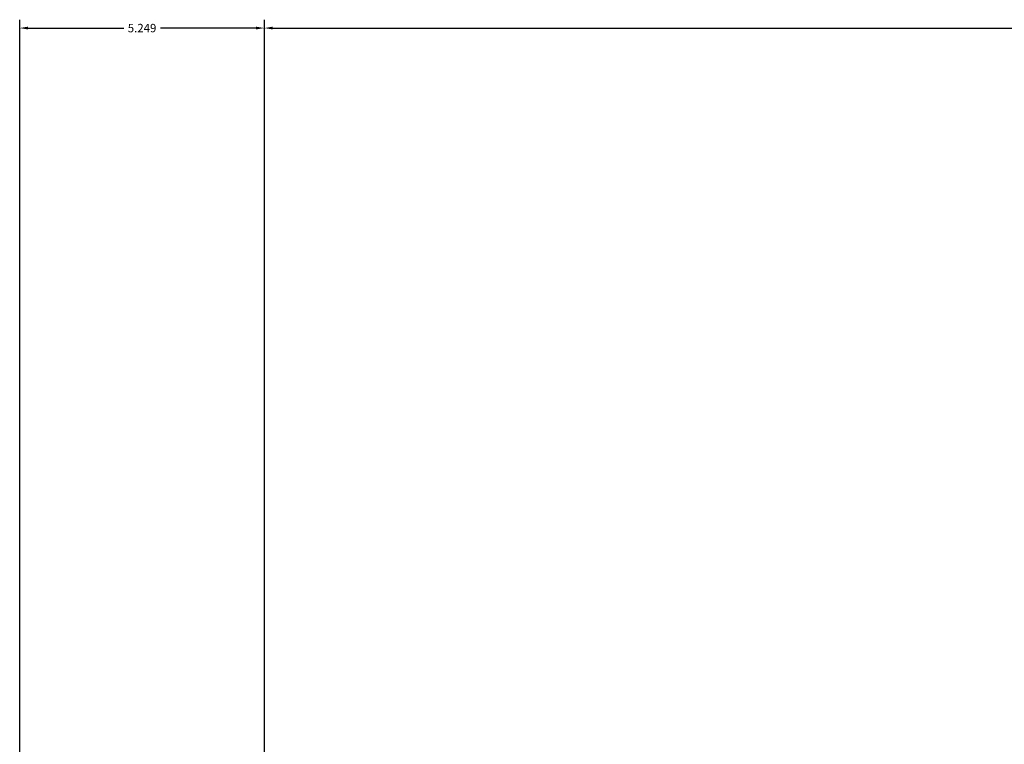
# Model space of a CAD drawing. Units: feet. Extents: x 2695 to 2912, y 795 to 1139.
# Tile 50 of 83: x 2711 to 2732, y 1123 to 1139. Entities that reach past the tile are written whole.
import ezdxf

# ---------------------------------------------------------------- set-up
doc = ezdxf.new("R2010")
doc.units = ezdxf.units.FT
doc.layers.add('A-ANNO-DIMS', color=2, linetype='Continuous', lineweight=18)
doc.styles.get("Standard").update_dxf_attribs({"font": 'arial.ttf'})
doc.dimstyles.get("Standard").update_dxf_attribs({"dimtxt": 0.18, "dimasz": 0.18, "dimexe": 0.18, "dimexo": 0.0625, "dimgap": 0.09, "dimtad": 0, "dimtih": 1, "dimtoh": 1, "dimdec": 1, "dimzin": 0, "dimdsep": 46, "dimlunit": 3, "dimtxsty": 'Standard', "dimcen": 0.09, "dimadec": 0, "dimazin": 0, "dimtfac": 1, "dimtdec": 1, "dimtofl": 0, "dimtmove": 0, "dimatfit": 3, "dimfxl": 1, "dimtolj": 1, "dimtzin": 0, "dimarcsym": 0})

# ---------------------------------------------------------------- blocks, each defined once
blk = doc.blocks.new('*D7')
at = {"layer": 'A-ANNO-DIMS', "color": 0, "lineweight": -2, "transparency": 16777216}
for p, q in [((2710.636, 1122.993), (2710.636, 1138.886)), ((2715.885, 1050.373), (2715.885, 1138.886)), ((2710.816, 1138.706), (2712.867, 1138.706)), ((2715.705, 1138.706), (2713.655, 1138.706))]:
    blk.add_line(p, q, dxfattribs=at)
at = {"layer": 'A-ANNO-DIMS', "color": 0, "transparency": 16777216}
for points in [[(2710.816, 1138.736), (2710.816, 1138.676), (2710.636, 1138.706)], [(2715.705, 1138.736), (2715.705, 1138.676), (2715.885, 1138.706)]]:
    blk.add_solid(points, dxfattribs=at)
at = {"layer": 'Defpoints', "color": 0, "transparency": 16777216}
for p in [(2715.885, 1138.706), (2710.636, 1122.931), (2715.885, 1050.311)]:
    blk.add_point(p, dxfattribs=at)
at = {"layer": 'A-ANNO-DIMS', "color": 0, "transparency": 16777216, "insert": (2713.261, 1138.706), "char_height": 0.18, "attachment_point": 5}
blk.add_mtext('\\A1;5.249', dxfattribs=at)
blk = doc.blocks.new('*D8')
at = {"layer": 'A-ANNO-DIMS', "color": 0, "lineweight": -2, "transparency": 16777216}
for p, q in [((2715.885, 1050.373), (2715.885, 1138.886)), ((2770.636, 1122.993), (2770.636, 1138.886)), ((2716.065, 1138.706), (2742.866, 1138.706)), ((2770.456, 1138.706), (2743.655, 1138.706))]:
    blk.add_line(p, q, dxfattribs=at)
at = {"layer": 'A-ANNO-DIMS', "color": 0, "transparency": 16777216}
for points in [[(2716.065, 1138.736), (2716.065, 1138.676), (2715.885, 1138.706)], [(2770.456, 1138.736), (2770.456, 1138.676), (2770.636, 1138.706)]]:
    blk.add_solid(points, dxfattribs=at)
at = {"layer": 'Defpoints', "color": 0, "transparency": 16777216}
for p in [(2770.636, 1138.706), (2770.636, 1122.931), (2715.885, 1050.311)]:
    blk.add_point(p, dxfattribs=at)
at = {"layer": 'A-ANNO-DIMS', "color": 0, "transparency": 16777216, "insert": (2743.261, 1138.706), "char_height": 0.18, "attachment_point": 5}
blk.add_mtext('\\A1;54.75', dxfattribs=at)

msp = doc.modelspace()

# ---------------------------------------------------------------- dimensions: what is measured, and where the dimension line sits
at = {"layer": 'A-ANNO-DIMS'}
for base, p1, p2, override, picture, middle in [((2715.8852, 1138.7056), (2710.6361, 1122.9306), (2715.8852, 1050.3105), {"dimdec": 3, "dimlfac": 1, "dimrnd": 0, "dimzin": 0, "dimdsep": 46, "dimlunit": 2}, '*D7', (2713.2606, 1138.7056)), ((2770.6361, 1138.7056), (2715.8852, 1050.3105), (2770.6361, 1122.9306), {"dimdec": 2, "dimlfac": 1, "dimrnd": 0, "dimzin": 0, "dimdsep": 46, "dimlunit": 2}, '*D8', (2743.2606, 1138.7056))]:
    dim = msp.add_linear_dim(base=base, p1=p1, p2=p2, dimstyle='Standard', override=override, dxfattribs=at)
    dim.commit()
    dim.dimension.update_dxf_attribs({"geometry": picture, "text_midpoint": middle})

doc.saveas('drawing.dxf')
